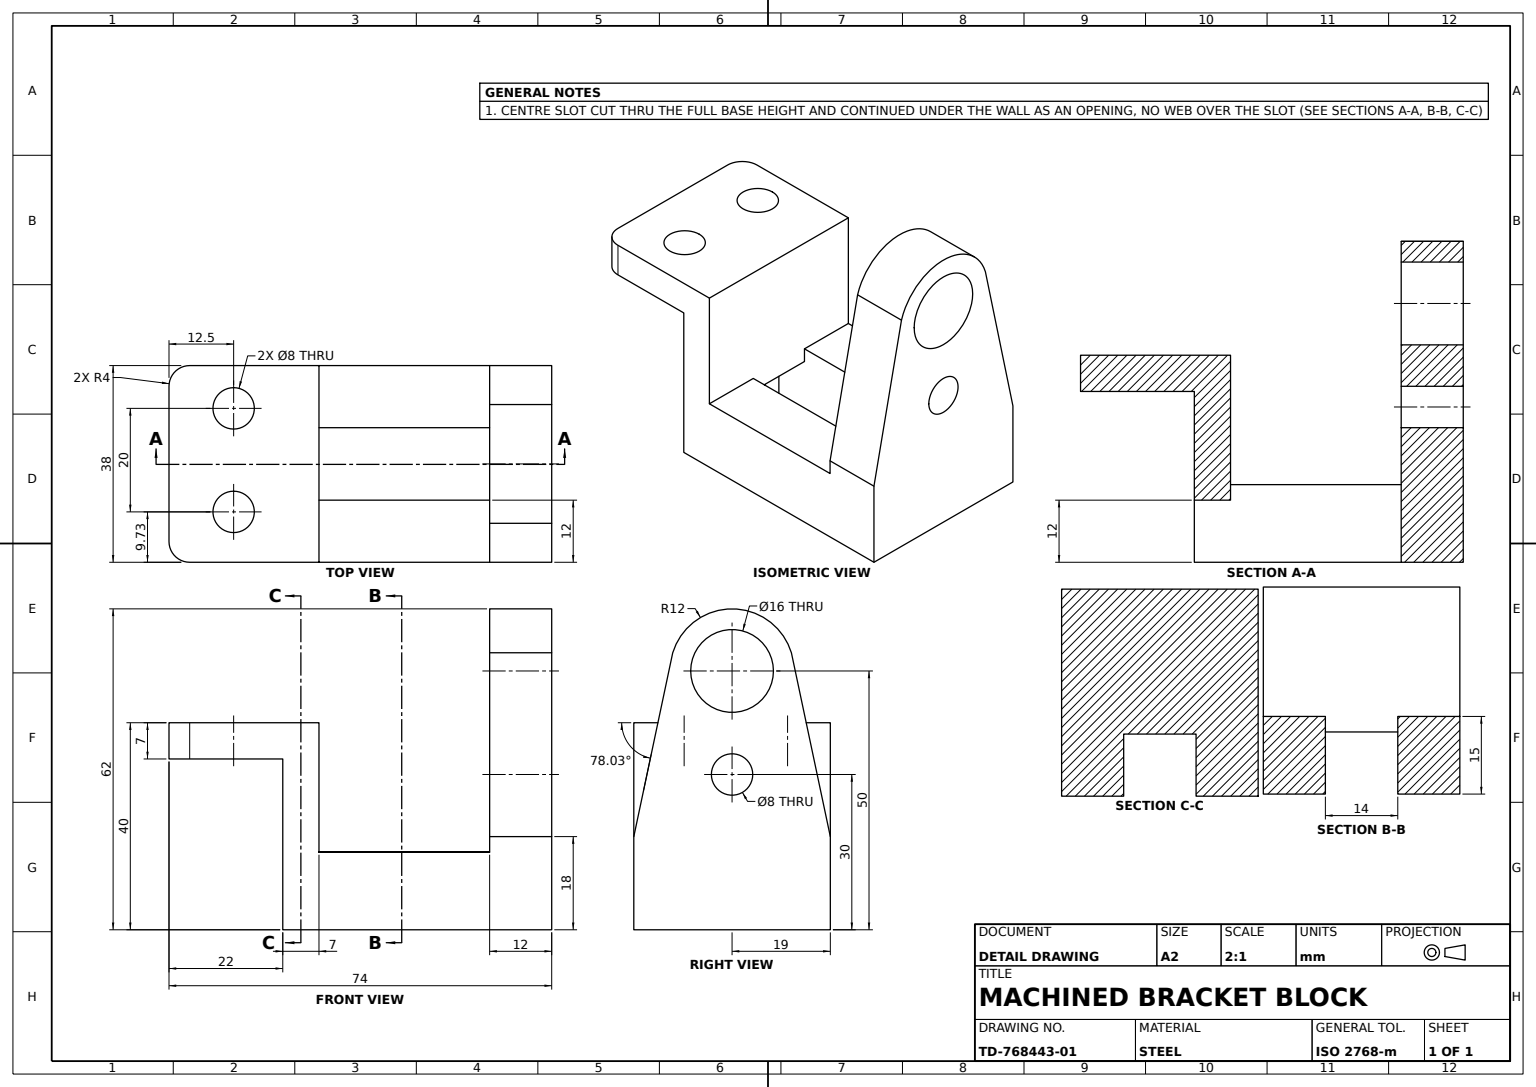
from build123d import *

# Parameters (mm, degrees)
BASE_BODY_DEPTH            = 38
UPRIGHT_LUG_DEPTH          = 12
CENTRE_SLOT_CUT_DEPTH      = 90.397986555
CENTRE_SLOT_CUT_DEPTH_BACK = 40
SIDE_WALL_SKETCH_W         = 7
SIDE_WALL_SKETCH_H         = 22
SIDE_WALL_DEPTH            = 38
TOP_FLANGE_DEPTH           = 7
SLOT_STEP_PAD_A_SKETCH_W   = 33
SLOT_STEP_PAD_A_SKETCH_H   = 12
SLOT_STEP_PAD_A_DEPTH      = 2
SLOT_STEP_PAD_B_SKETCH_W   = 33
SLOT_STEP_PAD_B_SKETCH_H   = 12
SLOT_STEP_PAD_B_DEPTH      = 2
FLANGE_HOLES_SKETCH_R      = 4
FLANGE_HOLES_2X_8_DEPTH    = 7
LUG_BORE_SKETCH_R          = 8
LUG_BORE_16_DEPTH          = 12
LUG_HOLE_SKETCH_R          = 4
LUG_HOLE_8_DEPTH           = 12
SLOT_STEP_BLOCK_A_SKETCH_W = 33
SLOT_STEP_BLOCK_A_SKETCH_H = 12
SLOT_STEP_BLOCK_A_DEPTH    = 5
SLOT_STEP_BLOCK_B_SKETCH_W = 33
SLOT_STEP_BLOCK_B_SKETCH_H = 12
SLOT_STEP_BLOCK_B_DEPTH    = 5


with BuildPart() as part:
    # Base Profile Sketch → Base Body (new body)
    with BuildSketch(Plane.XY):
        Polygon((0, 0), (52, 0), (52, 18), (40, 18), (40, 8), (12, 8), (7, 8), (7, 18), (0, 18), align=None)
    extrude(amount=BASE_BODY_DEPTH)

    # Upright Lug Sketch → Upright Lug (add)
    with BuildSketch(Plane(origin=(52, 0, 0), x_dir=(0, 0, -1), z_dir=(1, 0, 0))):
        with BuildLine():
            Line((-38, 18), (0, 18))
            Line((0, 18), (-7.527409318, 53.518474532))
            ThreePointArc((-7.527409318, 53.518474532), (-19, 62), (-30.472590682, 53.518474532))
            Line((-30.472590682, 53.518474532), (-38, 18))
        make_face()
    extrude(amount=-UPRIGHT_LUG_DEPTH)

    # Centre Slot Sketch → Centre Slot Cut (cut, two sides: drawn at the far end of the back side and taken through both)
    with BuildSketch(Plane.ZY.offset(-CENTRE_SLOT_CUT_DEPTH_BACK)):
        Polygon((26, -144.461890512), (26, 0), (26, 12), (12, 12), (12, 0), (12, -144.461890512), (12, -433.385671535), (26, -433.385671535), align=None)
    extrude(amount=CENTRE_SLOT_CUT_DEPTH + CENTRE_SLOT_CUT_DEPTH_BACK, mode=Mode.SUBTRACT)

    # Side Wall Sketch → Side Wall (add)
    with BuildSketch(Plane.XY.offset(38)):
        with Locations((3.5, 29)):
            Rectangle(SIDE_WALL_SKETCH_W, SIDE_WALL_SKETCH_H)
    extrude(amount=-SIDE_WALL_DEPTH)

    # Top Flange Sketch → Top Flange (add)
    with BuildSketch(Plane(origin=(0, 40, 0), x_dir=(1, 0, 0), z_dir=(0, 1, 0))):
        with BuildLine():
            Line((0, 0), (-18, 0))
            ThreePointArc((-18, 0), (-20.828427125, -1.171572875), (-22, -4))
            Line((-22, -4), (-22, -34))
            ThreePointArc((-22, -34), (-20.828427125, -36.828427125), (-18, -38))
            Line((-18, -38), (0, -38))
            Line((0, -38), (0, 0))
        make_face()
    extrude(amount=-TOP_FLANGE_DEPTH)

    # Slot Step Pad A Sketch → Slot Step Pad A (add)
    with BuildSketch(Plane(origin=(0, 8, 0), x_dir=(1, 0, 0), z_dir=(0, 1, 0))):
        with Locations((23.5, -32)):
            Rectangle(SLOT_STEP_PAD_A_SKETCH_W, SLOT_STEP_PAD_A_SKETCH_H)
    extrude(amount=SLOT_STEP_PAD_A_DEPTH)

    # Slot Step Pad B Sketch → Slot Step Pad B (add)
    with BuildSketch(Plane(origin=(0, 8, 0), x_dir=(1, 0, 0), z_dir=(0, 1, 0))):
        with Locations((23.5, -6)):
            Rectangle(SLOT_STEP_PAD_B_SKETCH_W, SLOT_STEP_PAD_B_SKETCH_H)
    extrude(amount=SLOT_STEP_PAD_B_DEPTH)

    # Flange Holes Sketch → Flange Holes 2xØ8 (cut)
    with BuildSketch(Plane(origin=(0, 40, 0), x_dir=(1, 0, 0), z_dir=(0, 1, 0))):
        with Locations(Location((-9.5, -8.266515029, 0), (0, 0, 270))):
            Circle(FLANGE_HOLES_SKETCH_R)
        with Locations(Location((-9.5, -28.266515029, 0), (0, 0, 270))):
            Circle(FLANGE_HOLES_SKETCH_R)
    extrude(amount=-FLANGE_HOLES_2X_8_DEPTH, mode=Mode.SUBTRACT)

    # Lug Bore Sketch → Lug Bore Ø16 (cut)
    with BuildSketch(Plane(origin=(52, 0, 0), x_dir=(0, 0, -1), z_dir=(1, 0, 0))):
        with Locations((-19, 50)):
            Circle(LUG_BORE_SKETCH_R)
    extrude(amount=-LUG_BORE_16_DEPTH, mode=Mode.SUBTRACT)

    # Lug Hole Sketch → Lug Hole Ø8 (cut)
    with BuildSketch(Plane(origin=(52, 0, 0), x_dir=(0, 0, -1), z_dir=(1, 0, 0))):
        with Locations((-19, 30)):
            Circle(LUG_HOLE_SKETCH_R)
    extrude(amount=-LUG_HOLE_8_DEPTH, mode=Mode.SUBTRACT)

    # Slot Step Block A Sketch → Slot Step Block A (add)
    with BuildSketch(Plane(origin=(0, 10, 0), x_dir=(1, 0, 0), z_dir=(0, 1, 0))):
        with Locations((23.5, -32)):
            Rectangle(SLOT_STEP_BLOCK_A_SKETCH_W, SLOT_STEP_BLOCK_A_SKETCH_H)
    extrude(amount=SLOT_STEP_BLOCK_A_DEPTH)

    # Slot Step Block B Sketch → Slot Step Block B (add)
    with BuildSketch(Plane(origin=(0, 10, 0), x_dir=(1, 0, 0), z_dir=(0, 1, 0))):
        with Locations((23.5, -6)):
            Rectangle(SLOT_STEP_BLOCK_B_SKETCH_W, SLOT_STEP_BLOCK_B_SKETCH_H)
    extrude(amount=SLOT_STEP_BLOCK_B_DEPTH)


solid = part.part
